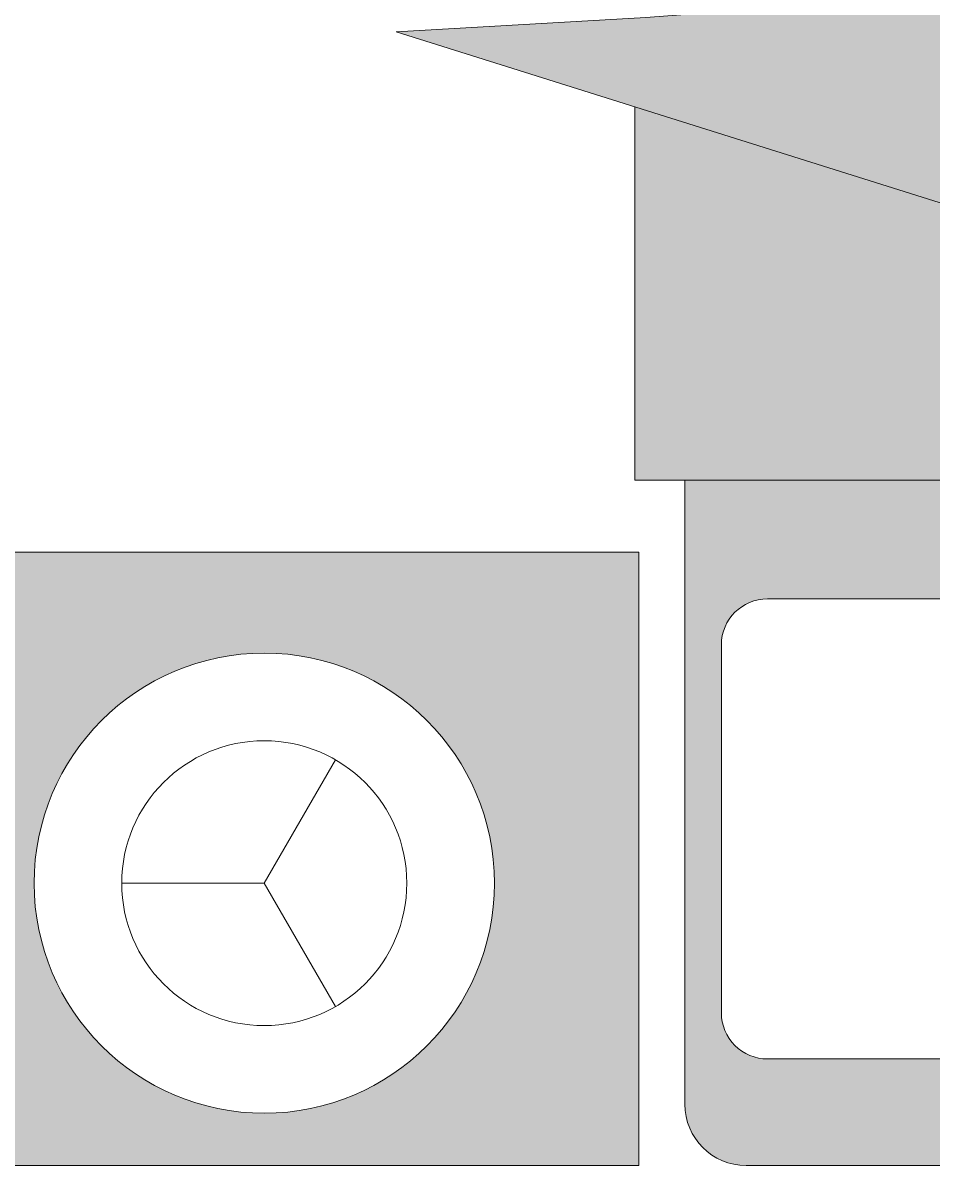
# Model space of a CAD drawing. Units: millimetres. Extents: x 27017497 to 27018854, y 7058029 to 7059154.
# Tile 69 of 91: x 27018367 to 27018390, y 7058144 to 7058174. Entities that reach past the tile are written whole.
import ezdxf

# ---------------------------------------------------------------- set-up
doc = ezdxf.new("R2010")
doc.units = ezdxf.units.MM
doc.layers.add('A-ANNO-DIMS', color=2, linetype='Continuous', lineweight=18)
doc.layers.add('A-FURN', color=8, linetype='Continuous', lineweight=18)
doc.layers.add('A-FURN-PATT', color=177, linetype='Continuous', lineweight=13, true_color=0x293189)
doc.styles.get("Standard").update_dxf_attribs({"font": 'arial.ttf'})
doc.dimstyles.get("Standard").update_dxf_attribs({"dimtxt": 0.18, "dimasz": 0.18, "dimexe": 0.18, "dimexo": 0.0625, "dimgap": 0.09, "dimtad": 0, "dimtih": 1, "dimtoh": 1, "dimdec": 4, "dimzin": 0, "dimdsep": 46, "dimtxsty": 'Standard', "dimcen": 0.09, "dimadec": 0, "dimazin": 0, "dimtfac": 1, "dimtdec": 4, "dimtofl": 0, "dimtmove": 0, "dimatfit": 3, "dimfxl": 1, "dimtolj": 1, "dimtzin": 0, "dimarcsym": 0})

# ---------------------------------------------------------------- blocks, each defined once
blk = doc.blocks.new('CAMMAT')
for p, q in [((0.61, -0.07), (-0.61, -0.07)), ((0.68, -0.07), (0.68, -0.47)), ((0.68, -0.07), (1.18, -0.07)), ((0.65, -0.11), (0.65, -0.51693)), ((0.59619, -0.1395), (0.05741, -0.1395)), ((0.62619, -0.1695), (0.62619, -0.4095)), ((0.92416, -0.2541), (0.87771, -0.17366)), ((0.92416, -0.2541), (0.87771, -0.33455)), ((0.92416, -0.2541), (1.01705, -0.2541)), ((0.59619, -0.4395), (0.05741, -0.4395)), ((0.68, -0.47), (1.18, -0.47)), ((-0.6904, -0.51693), (0.68256, -0.51693)), ((0.68256, -0.51693), (0.68256, -0.76028)), ((0.05354, -0.5623), (0.83824, -0.80928))]:
    blk.add_line(p, q)
blk.add_lwpolyline([(0.83824, -0.80928), (0.67535, -0.81849), (0.55218, -0.82799), (0.46223, -0.84058), (0.39901, -0.85906), (0.356, -0.8862), (0.3267, -0.92482), (0.3046, -0.9777), (0.28321, -1.04763)])
for radius in [0.15, 0.09289]:
    blk.add_circle((0.92416, -0.2541), radius)
for centre, radius, start, end in [((0.61, -0.11), 0.04, 0, 90), ((0.59619, -0.1695), 0.03, 360, 90), ((0.59619, -0.4095), 0.03, 270, 360)]:
    blk.add_arc(centre, radius, start, end)
blk = doc.blocks.new('*D47')
at = {"layer": 'A-ANNO-DIMS', "color": 0, "lineweight": -2, "transparency": 16777216}
for p, q in [((27017561.166, 7058294.35), (27017561.166, 7058028.6)), ((27018790.606, 7058294.35), (27018790.606, 7058028.6)), ((27017561.346, 7058028.78), (27018175.431, 7058028.78)), ((27018790.426, 7058028.78), (27018176.341, 7058028.78))]:
    blk.add_line(p, q, dxfattribs=at)
at = {"layer": 'A-ANNO-DIMS', "color": 0, "transparency": 16777216}
for points in [[(27017561.346, 7058028.81), (27017561.346, 7058028.75), (27017561.166, 7058028.78)], [(27018790.426, 7058028.81), (27018790.426, 7058028.75), (27018790.606, 7058028.78)]]:
    blk.add_solid(points, dxfattribs=at)
at = {"layer": 'Defpoints', "color": 0, "transparency": 16777216}
for p in [(27017561.166, 7058294.412), (27018790.606, 7058294.412), (27018790.606, 7058028.78)]:
    blk.add_point(p, dxfattribs=at)
at = {"layer": 'A-ANNO-DIMS', "color": 0, "transparency": 16777216, "insert": (27018175.886, 7058028.78), "char_height": 0.18, "attachment_point": 5}
blk.add_mtext('\\A1;1229.4', dxfattribs=at)
blk = doc.blocks.new('*D48')
at = {"layer": 'A-ANNO-DIMS', "color": 0, "lineweight": -2, "transparency": 16777216}
for p, q in [((27018463.498, 7058622.912), (27017497.536, 7058622.912)), ((27017497.716, 7058622.732), (27017497.716, 7058357.753)), ((27017497.716, 7058092.41), (27017497.716, 7058357.389)), ((27018555.129, 7058092.23), (27017497.536, 7058092.23))]:
    blk.add_line(p, q, dxfattribs=at)
at = {"layer": 'A-ANNO-DIMS', "color": 0, "transparency": 16777216}
for points in [[(27017497.686, 7058622.732), (27017497.746, 7058622.732), (27017497.716, 7058622.912)], [(27017497.686, 7058092.41), (27017497.746, 7058092.41), (27017497.716, 7058092.23)]]:
    blk.add_solid(points, dxfattribs=at)
at = {"layer": 'Defpoints', "color": 0, "transparency": 16777216}
for p in [(27018463.561, 7058622.912), (27017497.716, 7058092.23), (27018555.192, 7058092.23)]:
    blk.add_point(p, dxfattribs=at)
at = {"layer": 'A-ANNO-DIMS', "color": 0, "transparency": 16777216, "insert": (27017497.716, 7058357.571), "char_height": 0.18, "attachment_point": 5}
blk.add_mtext('\\A1;530.7', dxfattribs=at)

msp = doc.modelspace()

# ---------------------------------------------------------------- hatches: boundary and pattern name
at = {"layer": 'A-FURN-PATT'}
h = msp.add_hatch(color=256, dxfattribs=at)
h.dxf.hatch_style = 1
h.paths.add_polyline_path([(27018435.86, 7058218.784, 0.414214), (27018434.267, 7058220.377), (27018385.674, 7058220.377, 0.414214), (27018384.081, 7058218.784), (27018384.081, 7058174.59), (27018387.977, 7058174.891), (27018391.56, 7058175.393), (27018394.078, 7058176.128), (27018395.791, 7058177.21), (27018396.958, 7058178.748), (27018397.838, 7058180.854), (27018398.69, 7058183.639), (27018399.293, 7058180.835), (27018399.836, 7058178.594), (27018400.426, 7058176.691), (27018401.17, 7058174.899), (27018402.177, 7058172.991), (27018403.552, 7058170.741), (27018405.403, 7058167.922), (27018407.838, 7058164.308), (27018410.273, 7058167.922), (27018412.124, 7058170.741), (27018413.499, 7058172.991), (27018414.506, 7058174.899), (27018415.25, 7058176.691), (27018415.84, 7058178.594), (27018416.383, 7058180.835), (27018416.986, 7058183.639), (27018417.838, 7058180.854), (27018418.718, 7058178.748), (27018419.885, 7058177.21), (27018421.598, 7058176.128), (27018424.116, 7058175.393), (27018427.699, 7058174.891), (27018432.604, 7058174.513), (27018435.86, 7058174.329)])
h.paths.add_polyline_path([(27018439.093, 7058174.146), (27018432.604, 7058174.513), (27018427.699, 7058174.891), (27018424.116, 7058175.393), (27018421.598, 7058176.128), (27018419.885, 7058177.21), (27018418.718, 7058178.748), (27018417.838, 7058180.854), (27018416.986, 7058183.639), (27018416.383, 7058180.835), (27018415.84, 7058178.594), (27018415.25, 7058176.691), (27018414.506, 7058174.899), (27018413.499, 7058172.991), (27018412.124, 7058170.741), (27018410.273, 7058167.922), (27018407.838, 7058164.308)])
h.paths.add_polyline_path([(27018403.552, 7058170.741), (27018402.177, 7058172.991), (27018401.17, 7058174.899), (27018400.426, 7058176.691), (27018399.836, 7058178.594), (27018399.293, 7058180.835), (27018398.69, 7058183.639), (27018397.838, 7058180.854), (27018396.958, 7058178.748), (27018395.791, 7058177.21), (27018394.078, 7058176.128), (27018391.56, 7058175.393), (27018387.977, 7058174.891), (27018383.071, 7058174.513), (27018376.583, 7058174.146), (27018407.838, 7058164.308), (27018405.403, 7058167.922)])
h.paths.add_polyline_path([(27018437.469, 7058173.635), (27018407.838, 7058164.308), (27018382.784, 7058172.194), (27018382.784, 7058162.502), (27018437.469, 7058162.502)])
h.paths.add_polyline_path([(27018435.86, 7058162.502), (27018384.081, 7058162.502), (27018384.081, 7058146.294, 0.414214), (27018385.674, 7058144.7), (27018434.267, 7058144.7, 0.414214), (27018435.86, 7058146.294)])
h.paths.add_polyline_path([(27018407.684, 7058159.418, -0.41419), (27018408.879, 7058158.223), (27018408.879, 7058148.664, -0.414237), (27018407.684, 7058147.469), (27018386.224, 7058147.469, -0.41419), (27018385.029, 7058148.663), (27018385.029, 7058158.223, -0.414237), (27018386.224, 7058159.418)], flags=16)
h.paths.add_polyline_path([(27018411.821, 7058159.418), (27018433.28, 7058159.418, -0.41419), (27018434.475, 7058158.223), (27018434.475, 7058148.664, -0.414237), (27018433.28, 7058147.469), (27018411.821, 7058147.469, -0.414214), (27018410.626, 7058148.664), (27018410.626, 7058158.223, -0.414214)], flags=16)
h.paths.add_polyline_path([(27018382.886, 7058160.632), (27018362.971, 7058160.632), (27018362.971, 7058144.7), (27018382.886, 7058144.7)])
h.paths.add_polyline_path([(27018379.136, 7058152.033, -1), (27018367.187, 7058152.033, -1)], flags=16)
h.paths.add_polyline_path([(27018376.861, 7058152.033, -1), (27018369.461, 7058152.033, -1)], flags=0)
h.paths.add_polyline_path([(27018456.97, 7058160.632), (27018437.055, 7058160.632), (27018437.055, 7058144.7), (27018456.97, 7058144.7)])
h.paths.add_polyline_path([(27018453.028, 7058152.033, -1), (27018441.079, 7058152.033, -1)], flags=16)
h.paths.add_polyline_path([(27018450.754, 7058152.033, -1), (27018443.354, 7058152.033, -1)], flags=0)
h.paths.add_polyline_path([(27018434.475, 7058158.223, 0.41419), (27018433.28, 7058159.418), (27018411.821, 7058159.418, 0.414214), (27018410.626, 7058158.223), (27018410.626, 7058148.664, 0.414214), (27018411.821, 7058147.469), (27018433.28, 7058147.469, 0.414237), (27018434.475, 7058148.664)], flags=0)

# ---------------------------------------------------------------- block references
at = {"layer": 'A-FURN', "xscale": 39.82996475819422, "yscale": 39.82996475819422, "zscale": 39.82996475819422, "rotation": 180}
msp.add_blockref('CAMMAT', (27018409.97, 7058141.912), dxfattribs=at)

# ---------------------------------------------------------------- dimensions: what is measured, and where the dimension line sits
at = {"layer": 'A-ANNO-DIMS'}
dim = msp.add_linear_dim(base=(27017497.716, 7058092.23), p1=(27018463.561, 7058622.912), p2=(27018555.192, 7058092.23), angle=90, dimstyle='Standard', override={"dimdec": 1, "dimlfac": 1, "dimrnd": 0, "dimzin": 0, "dimdsep": 46, "dimlunit": 2}, dxfattribs=at)
dim.commit()
dim.dimension.update_dxf_attribs({"geometry": '*D48', "text_midpoint": (27017497.716, 7058357.571)})
dim = msp.add_linear_dim(base=(27018790.606, 7058028.78), p1=(27017561.166, 7058294.412), p2=(27018790.606, 7058294.412), dimstyle='Standard', override={"dimdec": 1, "dimlfac": 1, "dimrnd": 0, "dimzin": 0, "dimdsep": 46, "dimlunit": 2}, dxfattribs=at)
dim.commit()
dim.dimension.update_dxf_attribs({"geometry": '*D47', "text_midpoint": (27018175.886, 7058028.78)})

doc.saveas('drawing.dxf')
